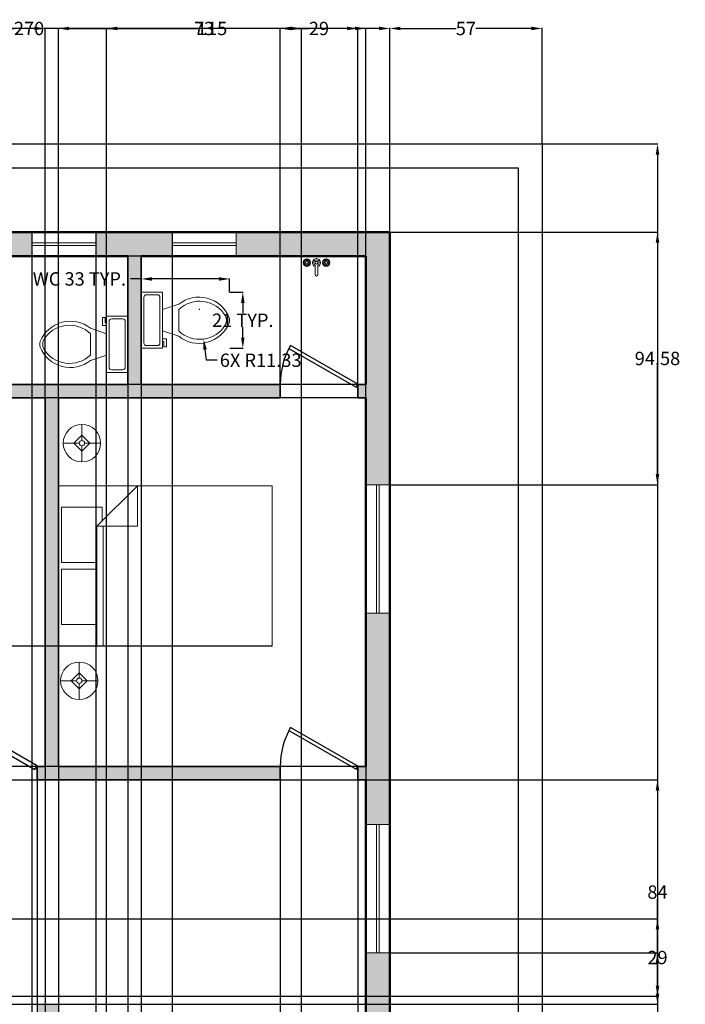
# Model space of a CAD drawing. Units: inches. Extents: x 882 to 1363, y 890 to 1847.
# Tile 9 of 9: x 1114 to 1363, y 1479 to 1847. Entities that reach past the tile are written whole.
import ezdxf

# ---------------------------------------------------------------- set-up
doc = ezdxf.new("R2010")
doc.units = ezdxf.units.IN
doc.header["$MEASUREMENT"] = 0
for name, color, linetype, lineweight in [('A-ANNO-DIMS', 2, 'Continuous', 18), ('C-PROP', 7, 'Continuous', 25), ('doors', 3, 'Continuous', 25), ('furniture', 10, 'Continuous', 18), ('inner wall', 50, 'Continuous', 35), ('outer wall', 40, 'Continuous', 50), ('sanitary', 231, 'Continuous', 18), ('ventilator', 130, 'Continuous', 18), ('windows', 226, 'Continuous', 18)]:
    doc.layers.add(name, color=color, linetype=linetype, lineweight=lineweight)
doc.layers.add('A-WALL-PATT', color=251, linetype='Continuous', lineweight=13, true_color=0x636466)
doc.styles.get("Standard").update_dxf_attribs({"font": 'arial.ttf'})
doc.dimstyles.get("Standard").update_dxf_attribs({"dimtxt": 5, "dimasz": 4, "dimexe": 0.18, "dimexo": 0.0625, "dimgap": 0.09, "dimtad": 0, "dimtih": 1, "dimtoh": 1, "dimdec": 1, "dimzin": 0, "dimdsep": 46, "dimlunit": 3, "dimtxsty": 'Standard', "dimcen": 0.09, "dimadec": 0, "dimazin": 0, "dimtfac": 1, "dimtdec": 1, "dimtofl": 0, "dimtmove": 0, "dimatfit": 3, "dimfxl": 1, "dimtolj": 1, "dimtzin": 0, "dimarcsym": 0})

# ---------------------------------------------------------------- blocks, each defined once
blk = doc.blocks.new('*U3')
for p, q in [((0, 0), (0, 6)), ((40, 0), (40, 6))]:
    blk.add_line(p, q)
blk.add_lwpolyline([(0, 0), (34.64, -20), (35.52, -18.48), (0.87, 1.52)], close=True)
blk.add_arc((0, 0), 40, 330, 0)
blk = doc.blocks.new('Toilet - top')
for p, q in [((9.5, -6), (9.5, -2)), ((-10, -8.5), (-8, -8.5)), ((-10, -9.5), (-10, -8.5)), ((-7, -9.5), (-10, -9.5)), ((-8, -8.5), (-8, -8)), ((-7, -8), (-7, -9.5)), ((-4, -8), (-6, -14)), ((4, -8), (6, -14)), ((4, -14), (-4, -14))]:
    blk.add_line(p, q)
blk.add_lwpolyline([(10.5, -8), (10.5, 0), (-10.5, 0), (-10.5, -8)], close=True)
for points in [[(-9.5, -2), (-9.5, -6)], [(8.5, -1), (-8.5, -1)], [(-8.5, -7), (8.5, -7)]]:
    blk.add_lwpolyline(points)
for centre, radius, start, end in [((-8.62, -1.88), 0.884, 81.8699, 188.1301), ((8.62, -1.88), 0.884, 351.8699, 98.1301), ((-8.62, -6.12), 0.884, 171.8699, 278.1301), ((8.62, -6.12), 0.884, 261.8699, 8.1301), ((3.52, -21.58), 12.17, 141.4691, 247.9714), ((4.2, -21.82), 11.33, 136.3677, 238.9468), ((-3.52, -21.58), 12.17, 292.0284, 38.5307), ((-4.2, -21.82), 11.33, 301.053, 43.6321), ((0, -27.88), 4, 245.7318, 294.2682), ((0, -29), 4, 254.8605, 285.1395)]:
    blk.add_arc(centre, radius, start, end)
blk = doc.blocks.new('Faucet - Bathroom top')
for p, q in [((-4.107, 0.125), (-4.375, 0.125)), ((-3.75, 0.4788), (-3.75, 0.75)), ((-3.5, 0.482), (-3.5, 0.75)), ((-3.1461, 0.125), (-2.875, 0.125)), ((3.143, 0.125), (2.875, 0.125)), ((3.5, 0.4788), (3.5, 0.75)), ((3.75, 0.482), (3.75, 0.75)), ((4.1039, 0.125), (4.375, 0.125)), ((-4.1039, -0.125), (-4.375, -0.125)), ((-3.75, -0.4821), (-3.75, -0.75)), ((-3.5, -0.4789), (-3.5, -0.75)), ((-3.143, -0.125), (-2.875, -0.125)), ((-0.5, -0.8639), (-0.5, -4.5)), ((0.5, -4.5), (0.5, -0.8631)), ((3.1461, -0.125), (2.875, -0.125)), ((3.5, -0.4821), (3.5, -0.75)), ((3.75, -0.4789), (3.75, -0.75)), ((4.107, -0.125), (4.375, -0.125))]:
    blk.add_line(p, q)
for centre, radius in [((-3.625, 0), 1.375), ((-4.625, 0), 0.2795), ((-3.625, 0), 0.5), ((-3.625, 1), 0.2795), ((-2.625, 0), 0.2795), ((0, 0), 0.5), ((3.625, 0), 1.375), ((2.625, 0), 0.2795), ((3.625, 0), 0.5), ((3.625, 1), 0.2795), ((4.625, 0), 0.2795), ((-3.625, -1), 0.2795), ((3.625, -1), 0.2795)]:
    blk.add_circle(centre, radius)
for centre, radius, start, end in [((-3.625, 0), 1, 105.2407, 164.2093), ((-3.625, 0), 1, 16.44125, 74.07887), ((0, 0), 1.5, 289.6514, 250.3603), ((0, 0), 1, 300.3431, 239.7554), ((3.625, 0), 1, 106.12, 164.0884), ((3.625, 0), 1, 16.23422, 73.90469), ((-3.625, 0), 1, 196.2342, 253.9047), ((-3.625, 0), 1, 286.12, 344.0884), ((3.625, 0), 1, 196.4413, 254.0789), ((3.625, 0), 1, 285.2407, 344.2093), ((0, -4.5), 0.5, 180, 0)]:
    blk.add_arc(centre, radius, start, end)
blk = doc.blocks.new('Bed - Queen')
for p, q in [((0, -80.00003), (0, 0)), ((0, 0), (59.99999, 0)), ((59.99999, 0), (59.99999, -80.00003)), ((7.99999, -1.2), (28.79998, -1.2)), ((7.99999, -14.4), (7.99999, -1.2)), ((28.79998, -1.2), (28.79998, -14.4)), ((31.19999, -1.2), (51.99999, -1.2)), ((31.19999, -14.4), (31.19999, -1.2)), ((51.99999, -1.2), (51.99999, -16.4)), ((0, -14.4), (44.8, -14.4)), ((59.99999, -29.6), (44.8, -14.4)), ((44.8, -14.4), (44.8, -29.6)), ((44.8, -16.8), (0, -16.8)), ((51.99999, -16.4), (46.79936, -16.4)), ((44.8, -29.6), (59.99999, -29.6)), ((59.99999, -80.00003), (0, -80.00003))]:
    blk.add_line(p, q)
blk = doc.blocks.new('Lamp - Table')
for p, q in [((0, 7), (0, 1)), ((-1, 0), (-7, 0)), ((0, 3), (-3, 0)), ((-3, 0), (0, -3)), ((3, 0), (0, 3)), ((0, -3), (3, 0)), ((1, 0), (7, 0)), ((0, -1), (0, -7))]:
    blk.add_line(p, q)
for radius in [7, 1]:
    blk.add_circle((0, 0), radius)
blk = doc.blocks.new('WIN-48IN-9IN')
for p, q in [((4, 0), (4, 48)), ((5, 0), (5, 48))]:
    blk.add_line(p, q)
blk.add_lwpolyline([(0, 48), (9, 48), (9, 0), (0, 0)], close=True)
blk = doc.blocks.new('VENT-24IN-9IN')
for p, q in [((24, 5), (0, 5)), ((24, 4), (0, 4))]:
    blk.add_line(p, q)
blk.add_lwpolyline([(0, 9), (24, 9), (24, 0), (0, 0)], close=True)
blk = doc.blocks.new('*D19')
at = {"layer": 'A-ANNO-DIMS', "color": 0, "lineweight": -2, "transparency": 16777216}
for p, q in [((1159.84, 1745.31), (1159.84, 1750.39)), ((1192.89, 1745.31), (1192.89, 1750.39)), ((1159.84, 1750.21), (1155.84, 1750.21)), ((1188.89, 1750.21), (1163.84, 1750.21))]:
    blk.add_line(p, q, dxfattribs=at)
at = {"layer": 'A-ANNO-DIMS', "color": 0, "transparency": 16777216}
for points in [[(1163.84, 1750.87), (1163.84, 1749.54), (1159.84, 1750.21)], [(1188.89, 1750.87), (1188.89, 1749.54), (1192.89, 1750.21)]]:
    blk.add_solid(points, dxfattribs=at)
at = {"layer": 'Defpoints', "color": 0, "transparency": 16777216}
for p in [(1159.84, 1750.21), (1159.84, 1745.25), (1192.89, 1745.25)]:
    blk.add_point(p, dxfattribs=at)
at = {"layer": 'A-ANNO-DIMS', "color": 0, "transparency": 16777216, "insert": (1136.69, 1750.21), "char_height": 5, "attachment_point": 5}
blk.add_mtext('\\A1;WC 33 TYP.', dxfattribs=at)
blk = doc.blocks.new('*D20')
at = {"layer": 'A-ANNO-DIMS', "color": 0, "lineweight": -2, "transparency": 16777216}
for p, q in [((1192.95, 1745.25), (1198.02, 1745.25)), ((1197.84, 1741.25), (1197.84, 1737.35)), ((1197.84, 1728.25), (1197.84, 1732.15)), ((1192.95, 1724.25), (1198.02, 1724.25))]:
    blk.add_line(p, q, dxfattribs=at)
at = {"layer": 'A-ANNO-DIMS', "color": 0, "transparency": 16777216}
for points in [[(1197.18, 1741.25), (1198.51, 1741.25), (1197.84, 1745.25)], [(1197.18, 1728.25), (1198.51, 1728.25), (1197.84, 1724.25)]]:
    blk.add_solid(points, dxfattribs=at)
at = {"layer": 'Defpoints', "color": 0, "transparency": 16777216}
for p in [(1192.89, 1745.25), (1197.84, 1745.25), (1192.89, 1724.25)]:
    blk.add_point(p, dxfattribs=at)
at = {"layer": 'A-ANNO-DIMS', "color": 0, "transparency": 16777216, "insert": (1197.84, 1734.75), "char_height": 5, "attachment_point": 5}
blk.add_mtext('\\A1;21 TYP.', dxfattribs=at)
blk = doc.blocks.new('*D34')
at = {"layer": 'A-ANNO-DIMS', "color": 0, "lineweight": -2, "transparency": 16777216}
for p, q in [((1309.9, 1800.75), (1353.22, 1800.75)), ((1353.04, 1796.75), (1353.04, 1371.39)), ((1353.04, 940.75), (1353.04, 1366.11)), ((1309.9, 936.75), (1353.22, 936.75))]:
    blk.add_line(p, q, dxfattribs=at)
at = {"layer": 'A-ANNO-DIMS', "color": 0, "transparency": 16777216}
for points in [[(1352.38, 1796.75), (1353.71, 1796.75), (1353.04, 1800.75)], [(1352.38, 940.75), (1353.71, 940.75), (1353.04, 936.75)]]:
    blk.add_solid(points, dxfattribs=at)
at = {"layer": 'Defpoints', "color": 0, "transparency": 16777216}
for p in [(1309.84, 1800.75), (1353.04, 1800.75), (1309.84, 936.75)]:
    blk.add_point(p, dxfattribs=at)
at = {"layer": 'A-ANNO-DIMS', "color": 0, "transparency": 16777216, "insert": (1353.04, 1368.75), "char_height": 5, "attachment_point": 5}
blk.add_mtext('\\A1;864', dxfattribs=at)
blk = doc.blocks.new('*D35')
at = {"layer": 'A-ANNO-DIMS', "color": 0, "lineweight": -2, "transparency": 16777216}
for p, q in [((1252.84, 1767.81), (1252.84, 1844.13)), ((1256.84, 1843.95), (1277.67, 1843.95)), ((1305.84, 1843.95), (1285.01, 1843.95)), ((1309.84, 1800.81), (1309.84, 1844.13))]:
    blk.add_line(p, q, dxfattribs=at)
at = {"layer": 'A-ANNO-DIMS', "color": 0, "transparency": 16777216}
for points in [[(1256.84, 1844.62), (1256.84, 1843.29), (1252.84, 1843.95)], [(1305.84, 1844.62), (1305.84, 1843.29), (1309.84, 1843.95)]]:
    blk.add_solid(points, dxfattribs=at)
at = {"layer": 'Defpoints', "color": 0, "transparency": 16777216}
for p in [(1252.84, 1843.95), (1309.84, 1800.75), (1252.84, 1767.75)]:
    blk.add_point(p, dxfattribs=at)
at = {"layer": 'A-ANNO-DIMS', "color": 0, "transparency": 16777216, "insert": (1281.34, 1843.95), "char_height": 5, "attachment_point": 5}
blk.add_mtext('\\A1;57', dxfattribs=at)
blk = doc.blocks.new('*D39')
at = {"layer": 'A-ANNO-DIMS', "color": 0, "lineweight": -2, "transparency": 16777216}
for p, q in [((982.84, 1767.81), (982.84, 1844.13)), ((986.84, 1843.95), (1112.19, 1843.95)), ((1248.84, 1843.95), (1123.49, 1843.95)), ((1252.84, 1767.81), (1252.84, 1844.13))]:
    blk.add_line(p, q, dxfattribs=at)
at = {"layer": 'A-ANNO-DIMS', "color": 0, "transparency": 16777216}
for points in [[(986.84, 1844.62), (986.84, 1843.29), (982.84, 1843.95)], [(1248.84, 1844.62), (1248.84, 1843.29), (1252.84, 1843.95)]]:
    blk.add_solid(points, dxfattribs=at)
at = {"layer": 'Defpoints', "color": 0, "transparency": 16777216}
for p in [(1252.84, 1843.95), (982.84, 1767.75), (1252.84, 1767.75)]:
    blk.add_point(p, dxfattribs=at)
at = {"layer": 'A-ANNO-DIMS', "color": 0, "transparency": 16777216, "insert": (1117.84, 1843.95), "char_height": 5, "attachment_point": 5}
blk.add_mtext('\\A1;270', dxfattribs=at)
blk = doc.blocks.new('*D41')
at = {"layer": 'A-ANNO-DIMS', "color": 0, "lineweight": -2, "transparency": 16777216}
for p, q in [((1069.84, 1758.69), (1069.84, 893.37)), ((1154.84, 1758.69), (1154.84, 893.37)), ((1073.84, 893.55), (1108.65, 893.55)), ((1150.84, 893.55), (1116.03, 893.55))]:
    blk.add_line(p, q, dxfattribs=at)
at = {"layer": 'A-ANNO-DIMS', "color": 0, "transparency": 16777216}
for points in [[(1073.84, 894.21), (1073.84, 892.88), (1069.84, 893.55)], [(1150.84, 894.21), (1150.84, 892.88), (1154.84, 893.55)]]:
    blk.add_solid(points, dxfattribs=at)
at = {"layer": 'Defpoints', "color": 0, "transparency": 16777216}
for p in [(1069.84, 1758.75), (1154.84, 1758.75), (1154.84, 893.55)]:
    blk.add_point(p, dxfattribs=at)
at = {"layer": 'A-ANNO-DIMS', "color": 0, "transparency": 16777216, "insert": (1112.34, 893.55), "char_height": 5, "attachment_point": 5}
blk.add_mtext('\\A1;85', dxfattribs=at)
blk = doc.blocks.new('*D42')
at = {"layer": 'A-ANNO-DIMS', "color": 0, "lineweight": -2, "transparency": 16777216}
for p, q in [((1159.84, 1710.69), (1159.84, 893.37)), ((1243.84, 1705.69), (1243.84, 893.37)), ((1163.84, 893.55), (1198.17, 893.55)), ((1239.84, 893.55), (1205.5, 893.55))]:
    blk.add_line(p, q, dxfattribs=at)
at = {"layer": 'A-ANNO-DIMS', "color": 0, "transparency": 16777216}
for points in [[(1163.84, 894.21), (1163.84, 892.88), (1159.84, 893.55)], [(1239.84, 894.21), (1239.84, 892.88), (1243.84, 893.55)]]:
    blk.add_solid(points, dxfattribs=at)
at = {"layer": 'Defpoints', "color": 0, "transparency": 16777216}
for p in [(1159.84, 1710.75), (1243.84, 1705.75), (1243.84, 893.55)]:
    blk.add_point(p, dxfattribs=at)
at = {"layer": 'A-ANNO-DIMS', "color": 0, "transparency": 16777216, "insert": (1201.84, 893.55), "char_height": 5, "attachment_point": 5}
blk.add_mtext('\\A1;84', dxfattribs=at)
blk = doc.blocks.new('*D43')
at = {"layer": 'A-ANNO-DIMS', "color": 0, "lineweight": -2, "transparency": 16777216}
for p, q in [((1243.78, 1758.75), (906.46, 1758.75)), ((906.64, 1754.75), (906.64, 1737.39)), ((906.64, 1714.75), (906.64, 1732.11)), ((1243.78, 1710.75), (906.46, 1710.75))]:
    blk.add_line(p, q, dxfattribs=at)
at = {"layer": 'A-ANNO-DIMS', "color": 0, "transparency": 16777216}
for points in [[(905.97, 1754.75), (907.3, 1754.75), (906.64, 1758.75)], [(905.97, 1714.75), (907.3, 1714.75), (906.64, 1710.75)]]:
    blk.add_solid(points, dxfattribs=at)
at = {"layer": 'Defpoints', "color": 0, "transparency": 16777216}
for p in [(1243.84, 1758.75), (906.64, 1710.75), (1243.84, 1710.75)]:
    blk.add_point(p, dxfattribs=at)
at = {"layer": 'A-ANNO-DIMS', "color": 0, "transparency": 16777216, "insert": (906.64, 1734.75), "char_height": 5, "attachment_point": 5}
blk.add_mtext('\\A1;48', dxfattribs=at)
blk = doc.blocks.new('*D44')
at = {"layer": 'A-ANNO-DIMS', "color": 0, "lineweight": -2, "transparency": 16777216}
for p, q in [((1243.78, 1705.75), (906.46, 1705.75)), ((906.64, 1701.75), (906.64, 1639.39)), ((906.64, 1571.75), (906.64, 1634.1)), ((1243.78, 1567.75), (906.46, 1567.75))]:
    blk.add_line(p, q, dxfattribs=at)
at = {"layer": 'A-ANNO-DIMS', "color": 0, "transparency": 16777216}
for points in [[(905.97, 1701.75), (907.3, 1701.75), (906.64, 1705.75)], [(905.97, 1571.75), (907.3, 1571.75), (906.64, 1567.75)]]:
    blk.add_solid(points, dxfattribs=at)
at = {"layer": 'Defpoints', "color": 0, "transparency": 16777216}
for p in [(1243.84, 1705.75), (906.64, 1567.75), (1243.84, 1567.75)]:
    blk.add_point(p, dxfattribs=at)
at = {"layer": 'A-ANNO-DIMS', "color": 0, "transparency": 16777216, "insert": (906.64, 1636.75), "char_height": 5, "attachment_point": 5}
blk.add_mtext('\\A1;138', dxfattribs=at)
blk = doc.blocks.new('*D45')
at = {"layer": 'A-ANNO-DIMS', "color": 0, "lineweight": -2, "transparency": 16777216}
for p, q in [((1128.84, 1567.81), (1128.84, 1844.13)), ((1132.84, 1843.95), (1180.94, 1843.95)), ((1239.84, 1843.95), (1191.74, 1843.95)), ((1243.84, 1567.81), (1243.84, 1844.13))]:
    blk.add_line(p, q, dxfattribs=at)
at = {"layer": 'A-ANNO-DIMS', "color": 0, "transparency": 16777216}
for points in [[(1132.84, 1844.62), (1132.84, 1843.29), (1128.84, 1843.95)], [(1239.84, 1844.62), (1239.84, 1843.29), (1243.84, 1843.95)]]:
    blk.add_solid(points, dxfattribs=at)
at = {"layer": 'Defpoints', "color": 0, "transparency": 16777216}
for p in [(1243.84, 1843.95), (1128.84, 1567.75), (1243.84, 1567.75)]:
    blk.add_point(p, dxfattribs=at)
at = {"layer": 'A-ANNO-DIMS', "color": 0, "transparency": 16777216, "insert": (1186.34, 1843.95), "char_height": 5, "attachment_point": 5}
blk.add_mtext('\\A1;115', dxfattribs=at)
blk = doc.blocks.new('*D46')
at = {"layer": 'A-ANNO-DIMS', "color": 0, "lineweight": -2, "transparency": 16777216}
for p, q in [((991.84, 1567.81), (991.84, 1844.13)), ((995.84, 1843.95), (1052.49, 1843.95)), ((1119.84, 1843.95), (1063.19, 1843.95)), ((1123.84, 1567.81), (1123.84, 1844.13))]:
    blk.add_line(p, q, dxfattribs=at)
at = {"layer": 'A-ANNO-DIMS', "color": 0, "transparency": 16777216}
for points in [[(995.84, 1844.62), (995.84, 1843.29), (991.84, 1843.95)], [(1119.84, 1844.62), (1119.84, 1843.29), (1123.84, 1843.95)]]:
    blk.add_solid(points, dxfattribs=at)
at = {"layer": 'Defpoints', "color": 0, "transparency": 16777216}
for p in [(1123.84, 1843.95), (991.84, 1567.75), (1123.84, 1567.75)]:
    blk.add_point(p, dxfattribs=at)
at = {"layer": 'A-ANNO-DIMS', "color": 0, "transparency": 16777216, "insert": (1057.84, 1843.95), "char_height": 5, "attachment_point": 5}
blk.add_mtext('\\A1;132', dxfattribs=at)
blk = doc.blocks.new('*D47')
at = {"layer": 'A-ANNO-DIMS', "color": 0, "lineweight": -2, "transparency": 16777216}
for p, q in [((1123.84, 1567.69), (1123.84, 893.37)), ((1128.84, 1567.69), (1128.84, 893.37)), ((1119.84, 893.55), (1115.84, 893.55)), ((1132.84, 893.55), (1136.84, 893.55))]:
    blk.add_line(p, q, dxfattribs=at)
at = {"layer": 'A-ANNO-DIMS', "color": 0, "transparency": 16777216}
for points in [[(1119.84, 894.21), (1119.84, 892.88), (1123.84, 893.55)], [(1132.84, 894.21), (1132.84, 892.88), (1128.84, 893.55)]]:
    blk.add_solid(points, dxfattribs=at)
at = {"layer": 'Defpoints', "color": 0, "transparency": 16777216}
for p in [(1123.84, 1567.75), (1128.84, 1567.75), (1128.84, 893.55)]:
    blk.add_point(p, dxfattribs=at)
at = {"layer": 'A-ANNO-DIMS', "color": 0, "transparency": 16777216, "insert": (1126.34, 893.55), "char_height": 5, "attachment_point": 5}
blk.add_mtext('\\A1;5', dxfattribs=at)
blk = doc.blocks.new('*D48')
at = {"layer": 'A-ANNO-DIMS', "color": 0, "lineweight": -2, "transparency": 16777216}
for p, q in [((1084.84, 1562.69), (1084.84, 893.37)), ((1120.84, 1562.69), (1120.84, 893.37)), ((1088.84, 893.55), (1099.17, 893.55)), ((1116.84, 893.55), (1106.51, 893.55))]:
    blk.add_line(p, q, dxfattribs=at)
at = {"layer": 'A-ANNO-DIMS', "color": 0, "transparency": 16777216}
for points in [[(1088.84, 894.21), (1088.84, 892.88), (1084.84, 893.55)], [(1116.84, 894.21), (1116.84, 892.88), (1120.84, 893.55)]]:
    blk.add_solid(points, dxfattribs=at)
at = {"layer": 'Defpoints', "color": 0, "transparency": 16777216}
for p in [(1084.84, 1562.75), (1120.84, 1562.75), (1120.84, 893.55)]:
    blk.add_point(p, dxfattribs=at)
at = {"layer": 'A-ANNO-DIMS', "color": 0, "transparency": 16777216, "insert": (1102.84, 893.55), "char_height": 5, "attachment_point": 5}
blk.add_mtext('\\A1;36', dxfattribs=at)
blk = doc.blocks.new('*D49')
at = {"layer": 'A-ANNO-DIMS', "color": 0, "lineweight": -2, "transparency": 16777216}
for p, q in [((1211.84, 1562.69), (1211.84, 893.37)), ((1240.84, 1562.69), (1240.84, 893.37)), ((1215.84, 893.55), (1222.62, 893.55)), ((1236.84, 893.55), (1230.06, 893.55))]:
    blk.add_line(p, q, dxfattribs=at)
at = {"layer": 'A-ANNO-DIMS', "color": 0, "transparency": 16777216}
for points in [[(1215.84, 894.21), (1215.84, 892.88), (1211.84, 893.55)], [(1236.84, 894.21), (1236.84, 892.88), (1240.84, 893.55)]]:
    blk.add_solid(points, dxfattribs=at)
at = {"layer": 'Defpoints', "color": 0, "transparency": 16777216}
for p in [(1211.84, 1562.75), (1240.84, 1562.75), (1240.84, 893.55)]:
    blk.add_point(p, dxfattribs=at)
at = {"layer": 'A-ANNO-DIMS', "color": 0, "transparency": 16777216, "insert": (1226.34, 893.55), "char_height": 5, "attachment_point": 5}
blk.add_mtext('\\A1;29', dxfattribs=at)
blk = doc.blocks.new('*D50')
at = {"layer": 'A-ANNO-DIMS', "color": 0, "lineweight": -2, "transparency": 16777216}
for p, q in [((1252.9, 1767.75), (1353.22, 1767.75)), ((1353.04, 1763.75), (1353.04, 1723.1)), ((1353.04, 1677.17), (1353.04, 1717.82)), ((1252.9, 1673.17), (1353.22, 1673.17))]:
    blk.add_line(p, q, dxfattribs=at)
at = {"layer": 'A-ANNO-DIMS', "color": 0, "transparency": 16777216}
for points in [[(1352.38, 1763.75), (1353.71, 1763.75), (1353.04, 1767.75)], [(1352.38, 1677.17), (1353.71, 1677.17), (1353.04, 1673.17)]]:
    blk.add_solid(points, dxfattribs=at)
at = {"layer": 'Defpoints', "color": 0, "transparency": 16777216}
for p in [(1252.84, 1767.75), (1252.84, 1673.17), (1353.04, 1673.17)]:
    blk.add_point(p, dxfattribs=at)
at = {"layer": 'A-ANNO-DIMS', "color": 0, "transparency": 16777216, "insert": (1353.04, 1720.46), "char_height": 5, "attachment_point": 5}
blk.add_mtext('\\A1;94.58', dxfattribs=at)
blk = doc.blocks.new('*D52')
at = {"layer": 'A-ANNO-DIMS', "color": 0, "lineweight": -2, "transparency": 16777216}
for p, q in [((1048.84, 1767.69), (1048.84, 893.37)), ((1118.86, 1767.69), (1118.86, 893.37)), ((1052.84, 893.55), (1075.83, 893.55)), ((1114.86, 893.55), (1091.87, 893.55))]:
    blk.add_line(p, q, dxfattribs=at)
at = {"layer": 'A-ANNO-DIMS', "color": 0, "transparency": 16777216}
for points in [[(1052.84, 894.21), (1052.84, 892.88), (1048.84, 893.55)], [(1114.86, 894.21), (1114.86, 892.88), (1118.86, 893.55)]]:
    blk.add_solid(points, dxfattribs=at)
at = {"layer": 'Defpoints', "color": 0, "transparency": 16777216}
for p in [(1048.84, 1767.75), (1118.86, 1767.75), (1118.86, 893.55)]:
    blk.add_point(p, dxfattribs=at)
at = {"layer": 'A-ANNO-DIMS', "color": 0, "transparency": 16777216, "insert": (1083.85, 893.55), "char_height": 5, "attachment_point": 5}
blk.add_mtext('\\A1;70.01', dxfattribs=at)
blk = doc.blocks.new('*D53')
at = {"layer": 'A-ANNO-DIMS', "color": 0, "lineweight": -2, "transparency": 16777216}
for p, q in [((1142.86, 1767.69), (1142.86, 893.37)), ((1171.41, 1767.69), (1171.41, 893.37)), ((1138.86, 893.55), (1134.86, 893.55)), ((1175.41, 893.55), (1179.41, 893.55))]:
    blk.add_line(p, q, dxfattribs=at)
at = {"layer": 'A-ANNO-DIMS', "color": 0, "transparency": 16777216}
for points in [[(1138.86, 894.21), (1138.86, 892.88), (1142.86, 893.55)], [(1175.41, 894.21), (1175.41, 892.88), (1171.41, 893.55)]]:
    blk.add_solid(points, dxfattribs=at)
at = {"layer": 'Defpoints', "color": 0, "transparency": 16777216}
for p in [(1142.86, 1767.75), (1171.41, 1767.75), (1171.41, 893.55)]:
    blk.add_point(p, dxfattribs=at)
at = {"layer": 'A-ANNO-DIMS', "color": 0, "transparency": 16777216, "insert": (1157.14, 893.55), "char_height": 5, "attachment_point": 5}
blk.add_mtext('\\A1;28.554', dxfattribs=at)
blk = doc.blocks.new('*D56')
at = {"layer": 'A-ANNO-DIMS', "color": 0, "lineweight": -2, "transparency": 16777216}
for p, q in [((991.9, 1562.75), (1353.22, 1562.75)), ((1353.04, 1558.75), (1353.04, 1523.39)), ((1353.04, 1482.75), (1353.04, 1518.11)), ((991.9, 1478.75), (1353.22, 1478.75))]:
    blk.add_line(p, q, dxfattribs=at)
at = {"layer": 'A-ANNO-DIMS', "color": 0, "transparency": 16777216}
for points in [[(1352.38, 1558.75), (1353.71, 1558.75), (1353.04, 1562.75)], [(1352.38, 1482.75), (1353.71, 1482.75), (1353.04, 1478.75)]]:
    blk.add_solid(points, dxfattribs=at)
at = {"layer": 'Defpoints', "color": 0, "transparency": 16777216}
for p in [(991.84, 1562.75), (991.84, 1478.75), (1353.04, 1478.75)]:
    blk.add_point(p, dxfattribs=at)
at = {"layer": 'A-ANNO-DIMS', "color": 0, "transparency": 16777216, "insert": (1353.04, 1520.75), "char_height": 5, "attachment_point": 5}
blk.add_mtext('\\A1;84', dxfattribs=at)
blk = doc.blocks.new('*D60')
at = {"layer": 'A-ANNO-DIMS', "color": 0, "lineweight": -2, "transparency": 16777216}
for p, q in [((1050.9, 1510.75), (1353.22, 1510.75)), ((1353.04, 1506.75), (1353.04, 1498.89)), ((1353.04, 1485.75), (1353.04, 1493.61)), ((1050.9, 1481.75), (1353.22, 1481.75))]:
    blk.add_line(p, q, dxfattribs=at)
at = {"layer": 'A-ANNO-DIMS', "color": 0, "transparency": 16777216}
for points in [[(1352.38, 1506.75), (1353.71, 1506.75), (1353.04, 1510.75)], [(1352.38, 1485.75), (1353.71, 1485.75), (1353.04, 1481.75)]]:
    blk.add_solid(points, dxfattribs=at)
at = {"layer": 'Defpoints', "color": 0, "transparency": 16777216}
for p in [(1050.84, 1510.75), (1050.84, 1481.75), (1353.04, 1481.75)]:
    blk.add_point(p, dxfattribs=at)
at = {"layer": 'A-ANNO-DIMS', "color": 0, "transparency": 16777216, "insert": (1353.04, 1496.25), "char_height": 5, "attachment_point": 5}
blk.add_mtext('\\A1;29', dxfattribs=at)
blk = doc.blocks.new('*D78')
at = {"layer": 'A-ANNO-DIMS', "color": 0, "lineweight": -2, "transparency": 16777216}
for p, q in [((1146.84, 1274.81), (1146.84, 1844.13)), ((1150.84, 1843.95), (1179.69, 1843.95)), ((1215.84, 1843.95), (1186.99, 1843.95)), ((1219.84, 1274.81), (1219.84, 1844.13))]:
    blk.add_line(p, q, dxfattribs=at)
at = {"layer": 'A-ANNO-DIMS', "color": 0, "transparency": 16777216}
for points in [[(1150.84, 1844.62), (1150.84, 1843.29), (1146.84, 1843.95)], [(1215.84, 1844.62), (1215.84, 1843.29), (1219.84, 1843.95)]]:
    blk.add_solid(points, dxfattribs=at)
at = {"layer": 'Defpoints', "color": 0, "transparency": 16777216}
for p in [(1219.84, 1843.95), (1146.84, 1274.75), (1219.84, 1274.75)]:
    blk.add_point(p, dxfattribs=at)
at = {"layer": 'A-ANNO-DIMS', "color": 0, "transparency": 16777216, "insert": (1183.34, 1843.95), "char_height": 5, "attachment_point": 5}
blk.add_mtext('\\A1;73', dxfattribs=at)
blk = doc.blocks.new('*D80')
at = {"layer": 'A-ANNO-DIMS', "color": 0, "lineweight": -2, "transparency": 16777216}
for p, q in [((1252.9, 1498.03), (1353.22, 1498.03)), ((1353.04, 1494.03), (1353.04, 1447.23)), ((1353.04, 1395.14), (1353.04, 1441.94)), ((1252.9, 1391.14), (1353.22, 1391.14))]:
    blk.add_line(p, q, dxfattribs=at)
at = {"layer": 'A-ANNO-DIMS', "color": 0, "transparency": 16777216}
for points in [[(1352.38, 1494.03), (1353.71, 1494.03), (1353.04, 1498.03)], [(1352.38, 1395.14), (1353.71, 1395.14), (1353.04, 1391.14)]]:
    blk.add_solid(points, dxfattribs=at)
at = {"layer": 'Defpoints', "color": 0, "transparency": 16777216}
for p in [(1252.84, 1498.03), (1353.04, 1498.03), (1252.84, 1391.14)]:
    blk.add_point(p, dxfattribs=at)
at = {"layer": 'A-ANNO-DIMS', "color": 0, "transparency": 16777216, "insert": (1353.04, 1444.58), "char_height": 5, "attachment_point": 5}
blk.add_mtext('\\A1;106.89', dxfattribs=at)
blk = doc.blocks.new('*D86')
at = {"layer": 'A-ANNO-DIMS', "color": 0, "lineweight": -2, "transparency": 16777216}
for p, q in [((1211.84, 1710.81), (1211.84, 1844.13)), ((1215.84, 1843.95), (1222.62, 1843.95)), ((1236.84, 1843.95), (1230.06, 1843.95)), ((1240.84, 1710.81), (1240.84, 1844.13))]:
    blk.add_line(p, q, dxfattribs=at)
at = {"layer": 'A-ANNO-DIMS', "color": 0, "transparency": 16777216}
for points in [[(1215.84, 1844.62), (1215.84, 1843.29), (1211.84, 1843.95)], [(1236.84, 1844.62), (1236.84, 1843.29), (1240.84, 1843.95)]]:
    blk.add_solid(points, dxfattribs=at)
at = {"layer": 'Defpoints', "color": 0, "transparency": 16777216}
for p in [(1240.84, 1843.95), (1211.84, 1710.75), (1240.84, 1710.75)]:
    blk.add_point(p, dxfattribs=at)
at = {"layer": 'A-ANNO-DIMS', "color": 0, "transparency": 16777216, "insert": (1226.34, 1843.95), "char_height": 5, "attachment_point": 5}
blk.add_mtext('\\A1;29', dxfattribs=at)
blk = doc.blocks.new('*D88')
at = {"layer": 'A-ANNO-DIMS', "color": 0, "lineweight": -2, "transparency": 16777216}
for p, q in [((1128.84, 1567.69), (1128.84, 893.37)), ((1211.84, 1562.69), (1211.84, 893.37)), ((1132.84, 893.55), (1166.66, 893.55)), ((1207.84, 893.55), (1174.01, 893.55))]:
    blk.add_line(p, q, dxfattribs=at)
at = {"layer": 'A-ANNO-DIMS', "color": 0, "transparency": 16777216}
for points in [[(1132.84, 894.21), (1132.84, 892.88), (1128.84, 893.55)], [(1207.84, 894.21), (1207.84, 892.88), (1211.84, 893.55)]]:
    blk.add_solid(points, dxfattribs=at)
at = {"layer": 'Defpoints', "color": 0, "transparency": 16777216}
for p in [(1128.84, 1567.75), (1211.84, 1562.75), (1211.84, 893.55)]:
    blk.add_point(p, dxfattribs=at)
at = {"layer": 'A-ANNO-DIMS', "color": 0, "transparency": 16777216, "insert": (1170.34, 893.55), "char_height": 5, "attachment_point": 5}
blk.add_mtext('\\A1;83', dxfattribs=at)
blk = doc.blocks.new('*D91')
at = {"layer": 'A-ANNO-DIMS', "color": 0, "lineweight": -2, "transparency": 16777216}
for p, q in [((1208.78, 1612.84), (906.46, 1612.84)), ((906.64, 1608.84), (906.64, 1592.94)), ((906.64, 1571.75), (906.64, 1587.65)), ((1211.78, 1567.75), (906.46, 1567.75))]:
    blk.add_line(p, q, dxfattribs=at)
at = {"layer": 'A-ANNO-DIMS', "color": 0, "transparency": 16777216}
for points in [[(905.97, 1608.84), (907.3, 1608.84), (906.64, 1612.84)], [(905.97, 1571.75), (907.3, 1571.75), (906.64, 1567.75)]]:
    blk.add_solid(points, dxfattribs=at)
at = {"layer": 'Defpoints', "color": 0, "transparency": 16777216}
for p in [(1208.84, 1612.84), (906.64, 1567.75), (1211.84, 1567.75)]:
    blk.add_point(p, dxfattribs=at)
at = {"layer": 'A-ANNO-DIMS', "color": 0, "transparency": 16777216, "insert": (906.64, 1590.29), "char_height": 5, "attachment_point": 5}
blk.add_mtext('\\A1;45.09', dxfattribs=at)
blk = doc.blocks.new('*D96')
at = {"layer": 'A-ANNO-DIMS', "color": 0, "lineweight": -2, "transparency": 16777216}
for p, q in [((1181.57, 1738.95), (1181.75, 1738.95)), ((1181.66, 1738.86), (1181.66, 1739.04)), ((1184.23, 1719.79), (1183.7, 1723.76)), ((1188.23, 1719.79), (1184.23, 1719.79))]:
    blk.add_line(p, q, dxfattribs=at)
at = {"layer": 'A-ANNO-DIMS', "color": 0, "transparency": 16777216}
blk.add_solid([(1184.36, 1723.85), (1183.04, 1723.67), (1183.17, 1727.72)], dxfattribs=at)
at = {"layer": 'Defpoints', "color": 0, "transparency": 16777216}
for p in [(1181.66, 1738.95), (1183.17, 1727.72)]:
    blk.add_point(p, dxfattribs=at)
at = {"layer": 'A-ANNO-DIMS', "color": 0, "transparency": 16777216, "insert": (1204.54, 1719.79), "char_height": 5, "attachment_point": 5}
blk.add_mtext('\\A1;6X R11.33', dxfattribs=at)

msp = doc.modelspace()

# ---------------------------------------------------------------- hatches: boundary and pattern name
at = {"layer": 'A-WALL-PATT'}
h = msp.add_hatch(color=256, dxfattribs=at)
h.dxf.hatch_style = 1
h.paths.add_polyline_path([(1050.8388, 1481.7495), (1050.8388, 1478.7495), (1084.8388, 1478.7495), (1084.8388, 1473.7495), (991.8388, 1473.7495), (991.8388, 1361.0778), (982.8388, 1361.0778), (982.8388, 1556.1531), (991.8388, 1556.1531), (991.8388, 1478.7495), (1045.8388, 1478.7495), (1045.8388, 1481.7479), (1045.4161, 1481.7477), (1030.9055, 1506.8563), (1032.004, 1507.4911), (1046.5146, 1482.3825), (1045.4161, 1481.7477), (1045.8388, 1481.7479), (1045.8388, 1481.7495)])
h.paths.add_polyline_path([(1128.8388, 1478.7495), (1120.8388, 1478.7495), (1120.8388, 1473.7495), (1123.8388, 1473.7495), (1123.8388, 1353.7495), (991.8388, 1353.7495), (991.8388, 1361.0778), (982.8388, 1361.0778), (982.8388, 1337.3333), (991.8388, 1337.3333), (991.8388, 1348.7495), (1128.8388, 1348.7495)])
h.paths.add_polyline_path([(1118.8585, 1767.7495), (1048.8447, 1767.7495), (1048.8447, 1758.7495), (1064.8388, 1758.7495), (1069.8388, 1758.7495), (1118.8585, 1758.7495)])
h.paths.add_polyline_path([(1171.4129, 1767.7495), (1142.8585, 1767.7495), (1142.8585, 1758.7495), (1154.8388, 1758.7495), (1154.8388, 1710.7495), (1069.8388, 1710.7495), (1069.8388, 1713.7495), (1064.8388, 1713.7495), (1064.8388, 1705.7495), (1123.8388, 1705.7495), (1123.8388, 1567.7495), (1120.8388, 1567.7495), (1120.8388, 1562.7495), (1123.8388, 1562.7495), (1211.8388, 1562.7495), (1211.8388, 1567.7495), (1128.8388, 1567.7495), (1128.8388, 1705.7495), (1211.8388, 1705.7495), (1211.8388, 1710.7495), (1159.8388, 1710.7495), (1159.8388, 1758.7495), (1171.4129, 1758.7495)])
h.paths.add_polyline_path([(1252.8388, 1767.7495), (1195.4129, 1767.7495), (1195.4129, 1758.7495), (1243.8388, 1758.7495), (1243.8388, 1710.7495), (1240.8388, 1710.7495), (1240.8388, 1706.4648), (1240.8388, 1705.7495), (1243.8388, 1705.7495), (1243.8388, 1673.1735), (1252.8388, 1673.1735)])
h.paths.add_polyline_path([(1252.8388, 1625.1735), (1243.8388, 1625.1735), (1243.8388, 1567.7495), (1240.8388, 1567.7495), (1240.8388, 1562.7495), (1243.8388, 1562.7495), (1243.8388, 1546.029), (1252.8388, 1546.029)])
h.paths.add_polyline_path([(1252.8388, 1498.029), (1243.8388, 1498.029), (1243.8388, 1391.1399), (1252.8388, 1391.1399)])
h.paths.add_polyline_path([(1252.8388, 1179.8561), (1243.8388, 1179.8561), (1243.8388, 1149.7495), (1219.8388, 1149.7495), (1219.8388, 1145.3111), (1219.8388, 1144.7495), (1252.8388, 1144.7495)])
h.paths.add_polyline_path([(1252.8388, 1277.7495), (1243.8388, 1277.7495), (1243.8388, 1274.7495), (1219.8388, 1274.7495), (1219.8388, 1269.7495), (1243.8388, 1269.7495), (1243.8388, 1227.8561), (1252.8388, 1227.8561)])
h.paths.add_polyline_path([(1252.8388, 1343.1399), (1243.8388, 1343.1399), (1243.8388, 1313.7495), (1248.3388, 1313.7495), (1252.8388, 1313.7495)])
h.paths.add_polyline_path([(1146.8388, 1274.7495), (1112.8388, 1274.7495), (1112.8388, 1106.7495), (1106.7761, 1106.7495), (1106.7761, 1101.7495), (1117.8388, 1101.7495), (1117.8388, 1144.7495), (1159.8388, 1144.7495), (1159.8388, 1149.7495), (1117.8388, 1149.7495), (1117.8388, 1269.7495), (1146.8388, 1269.7495)])
h = msp.add_hatch(color=256, dxfattribs=at)
h.dxf.hatch_style = 1
h.paths.add_polyline_path([(1069.8388, 1758.7495), (1118.8585, 1758.7495), (1118.8585, 1767.7495), (1048.8447, 1767.7495), (1048.8447, 1758.7495), (1064.8388, 1758.7495), (1064.8388, 1742.7495), (1069.8388, 1742.7495)])

# ---------------------------------------------------------------- linework, layer by layer
at = {"layer": 'C-PROP'}
for points in [[(949.8388, 1800.7495), (1309.8388, 1800.7495), (1309.8388, 936.7495), (949.8388, 936.7495)], [(958.8388, 1791.7495), (1300.8388, 1791.7495), (1300.8388, 945.7495), (958.8388, 945.7495)]]:
    msp.add_lwpolyline(points, close=True, dxfattribs=at)
at = {"layer": 'inner wall'}
for p, q in [((1154.8388, 1758.7495), (1154.8388, 1710.7495)), ((1159.8388, 1758.7495), (1159.8388, 1710.7495)), ((1069.8388, 1710.7495), (1154.8388, 1710.7495)), ((1159.8388, 1710.7495), (1211.8388, 1710.7495)), ((1211.8388, 1710.7495), (1211.8388, 1705.7495)), ((1240.8388, 1710.7495), (1240.8388, 1705.7495)), ((1240.8388, 1710.7495), (1243.8388, 1710.7495)), ((1064.8388, 1705.7495), (1123.8388, 1705.7495)), ((1123.8388, 1567.7495), (1123.8388, 1705.7495)), ((1128.8388, 1705.7495), (1211.8388, 1705.7495)), ((1128.8388, 1567.7495), (1128.8388, 1705.7495)), ((1240.8388, 1705.7495), (1243.8388, 1705.7495)), ((1120.8388, 1562.7495), (1120.8388, 1567.7495)), ((1120.8388, 1567.7495), (1123.8388, 1567.7495)), ((1128.8388, 1567.7495), (1211.8388, 1567.7495)), ((1211.8388, 1567.7495), (1211.8388, 1562.7495)), ((1240.8388, 1567.7495), (1240.8388, 1562.7495)), ((1240.8388, 1567.7495), (1243.8388, 1567.7495)), ((1120.8388, 1562.7495), (1123.8388, 1562.7495)), ((1123.8388, 1562.7495), (1211.8388, 1562.7495)), ((1240.8388, 1562.7495), (1243.8388, 1562.7495))]:
    msp.add_line(p, q, dxfattribs=at)
at = {"layer": 'outer wall'}
for p, q in [((982.8388, 1767.7495), (1252.8388, 1767.7495)), ((1252.8388, 1767.7495), (1252.8388, 1313.7495)), ((1069.8388, 1758.7495), (1154.8388, 1758.7495)), ((1159.8388, 1758.7495), (1243.8388, 1758.7495)), ((1243.8388, 1758.7495), (1243.8388, 1710.7495)), ((1243.8388, 1705.7495), (1243.8388, 1567.7495)), ((1243.8388, 1562.7495), (1243.8388, 1313.7495))]:
    msp.add_line(p, q, dxfattribs=at)
at = {"layer": 'ventilator'}
for p, q in [((1142.8585, 1763.7495), (1118.8585, 1763.7495)), ((1142.8585, 1762.7495), (1118.8585, 1762.7495))]:
    msp.add_line(p, q, dxfattribs=at)
msp.add_lwpolyline([(1118.8585, 1767.7495), (1142.8585, 1767.7495), (1142.8585, 1758.7495), (1118.8585, 1758.7495)], close=True, dxfattribs=at)

# ---------------------------------------------------------------- block references
at = {"layer": 'doors', "rotation": 180}
for p, xscale, yscale, zscale in [((1240.8388, 1710.8148), 0.725, 0.725, 0.725), ((1120.8388, 1567.9495), 0.9, 0.9, 0.9), ((1240.8388, 1567.8122), 0.725, 0.725, 0.725)]:
    msp.add_blockref('*U3', p, dxfattribs=dict(at, xscale=xscale, yscale=yscale, zscale=zscale))
at = {"layer": 'furniture'}
for p in [(1137.6388, 1688.7495), (1136.6388, 1599.8306)]:
    msp.add_blockref('Lamp - Table', p, dxfattribs=at)
at = {"layer": 'furniture', "rotation": 90}
msp.add_blockref('Bed - Queen', (1128.8388, 1612.8355), dxfattribs=at)
at = {"layer": 'sanitary'}
msp.add_blockref('Faucet - Bathroom top', (1225.4236, 1756.3037), dxfattribs=at)
for p, rotation in [((1159.8388, 1734.7495), 90), ((1154.8388, 1725.7299), 270)]:
    msp.add_blockref('Toilet - top', p, dxfattribs=dict(at, rotation=rotation))
at = {"layer": 'ventilator'}
msp.add_blockref('VENT-24IN-9IN', (1171.413, 1758.75), dxfattribs=at)
at = {"layer": 'windows'}
for p in [(1243.839, 1625.1738), (1243.839, 1498.0292)]:
    msp.add_blockref('WIN-48IN-9IN', p, dxfattribs=at)

# ---------------------------------------------------------------- dimensions: what is measured, and where the dimension line sits
at = {"layer": 'A-ANNO-DIMS'}
for base, p1, p2, override, picture, middle in [((1252.8388, 1843.953), (982.8388, 1767.7495), (1252.8388, 1767.7495), {"dimdec": 0, "dimlfac": 1, "dimrnd": 0, "dimzin": 0, "dimdsep": 46, "dimlunit": 2}, '*D39', (1117.8388, 1843.953)), ((1123.8388, 1843.953), (991.8388, 1567.7495), (1123.8388, 1567.7495), {"dimdec": 0, "dimlfac": 1, "dimrnd": 0, "dimzin": 0, "dimdsep": 46, "dimlunit": 2}, '*D46', (1057.8388, 1843.953)), ((1243.8388, 1843.953), (1128.8388, 1567.7495), (1243.8388, 1567.7495), {"dimdec": 0, "dimlfac": 1, "dimrnd": 0, "dimzin": 0, "dimdsep": 46, "dimlunit": 2}, '*D45', (1186.3388, 1843.953)), ((1219.8388, 1843.953), (1146.8388, 1274.7495), (1219.8388, 1274.7495), {"dimdec": 0, "dimlfac": 1, "dimrnd": 0, "dimzin": 0, "dimdsep": 46, "dimlunit": 2}, '*D78', (1183.3388, 1843.953)), ((1240.8388, 1843.953), (1211.8388, 1710.7495), (1240.8388, 1710.7495), {"dimdec": 0, "dimlfac": 1, "dimrnd": 0, "dimzin": 0, "dimdsep": 46, "dimlunit": 2}, '*D86', (1226.3388, 1843.953)), ((1252.8388, 1843.953), (1309.8388, 1800.7495), (1252.8388, 1767.7495), {"dimdec": 0, "dimlfac": 1, "dimrnd": 0, "dimzin": 0, "dimdsep": 46, "dimlunit": 2}, '*D35', (1281.3388, 1843.953)), ((1118.8585, 893.546), (1048.8447, 1767.7495), (1118.8585, 1767.7495), {"dimdec": 2, "dimlfac": 1, "dimrnd": 0, "dimzin": 0, "dimdsep": 46, "dimlunit": 2}, '*D52', (1083.8516, 893.546)), ((1171.4129, 893.546), (1142.8585, 1767.7495), (1171.4129, 1767.7495), {"dimdec": 3, "dimlfac": 1, "dimrnd": 0, "dimzin": 0, "dimdsep": 46, "dimlunit": 2}, '*D53', (1157.1357, 893.546)), ((1154.8388, 893.546), (1069.8388, 1758.7495), (1154.8388, 1758.7495), {"dimdec": 0, "dimlfac": 1, "dimrnd": 0, "dimzin": 0, "dimdsep": 46, "dimlunit": 2}, '*D41', (1112.3388, 893.546)), ((1243.8388, 893.546), (1159.8388, 1710.7495), (1243.8388, 1705.7495), {"dimdec": 0, "dimlfac": 1, "dimrnd": 0, "dimzin": 0, "dimdsep": 46, "dimlunit": 2}, '*D42', (1201.8388, 893.546)), ((1128.8388, 893.546), (1123.8388, 1567.7495), (1128.8388, 1567.7495), {"dimdec": 0, "dimlfac": 1, "dimrnd": 0, "dimzin": 0, "dimdsep": 46, "dimlunit": 2}, '*D47', (1126.3388, 893.546)), ((1211.8388, 893.546), (1128.8388, 1567.7495), (1211.8388, 1562.7495), {"dimdec": 0, "dimlfac": 1, "dimrnd": 0, "dimzin": 0, "dimdsep": 46, "dimlunit": 2}, '*D88', (1170.3388, 893.546)), ((1120.8388, 893.546), (1084.8388, 1562.7495), (1120.8388, 1562.7495), {"dimdec": 0, "dimlfac": 1, "dimrnd": 0, "dimzin": 0, "dimdsep": 46, "dimlunit": 2}, '*D48', (1102.8388, 893.546)), ((1240.8388, 893.546), (1211.8388, 1562.7495), (1240.8388, 1562.7495), {"dimdec": 0, "dimlfac": 1, "dimrnd": 0, "dimzin": 0, "dimdsep": 46, "dimlunit": 2}, '*D49', (1226.3388, 893.546))]:
    dim = msp.add_linear_dim(base=base, p1=p1, p2=p2, dimstyle='Standard', override=override, dxfattribs=at)
    dim.commit()
    dim.dimension.update_dxf_attribs({"geometry": picture, "text_midpoint": middle})
for base, p1, p2, override, picture, middle in [((1353.0423, 1800.7495), (1309.8388, 936.7495), (1309.8388, 1800.7495), {"dimdec": 0, "dimlfac": 1, "dimrnd": 0, "dimzin": 0, "dimdsep": 46, "dimlunit": 2}, '*D34', (1353.0423, 1368.7495)), ((1353.0423, 1673.1735), (1252.8388, 1767.7495), (1252.8388, 1673.1735), {"dimdec": 2, "dimlfac": 1, "dimrnd": 0, "dimzin": 0, "dimdsep": 46, "dimlunit": 2}, '*D50', (1353.0423, 1720.4615)), ((906.6353, 1710.7495), (1243.8388, 1758.7495), (1243.8388, 1710.7495), {"dimdec": 0, "dimlfac": 1, "dimrnd": 0, "dimzin": 0, "dimdsep": 46, "dimlunit": 2}, '*D43', (906.6353, 1734.7495)), ((906.6353, 1567.7495), (1243.8388, 1705.7495), (1243.8388, 1567.7495), {"dimdec": 0, "dimlfac": 1, "dimrnd": 0, "dimzin": 0, "dimdsep": 46, "dimlunit": 2}, '*D44', (906.6353, 1636.7495)), ((906.6353, 1567.7495), (1208.8389, 1612.8355), (1211.8388, 1567.7495), {"dimdec": 2, "dimlfac": 1, "dimrnd": 0, "dimzin": 0, "dimdsep": 46, "dimlunit": 2}, '*D91', (906.6353, 1590.2925)), ((1353.0423, 1478.7495), (991.8388, 1562.7495), (991.8388, 1478.7495), {"dimdec": 0, "dimlfac": 1, "dimrnd": 0, "dimzin": 0, "dimdsep": 46, "dimlunit": 2}, '*D56', (1353.0423, 1520.7495)), ((1353.0423, 1481.7495), (1050.8388, 1510.7495), (1050.8388, 1481.7495), {"dimdec": 0, "dimlfac": 1, "dimrnd": 0, "dimzin": 0, "dimdsep": 46, "dimlunit": 2}, '*D60', (1353.0423, 1496.2495)), ((1353.0423, 1498.029), (1252.8388, 1391.1399), (1252.8388, 1498.029), {"dimdec": 2, "dimlfac": 1, "dimrnd": 0, "dimzin": 0, "dimdsep": 46, "dimlunit": 2}, '*D80', (1353.0423, 1444.5844))]:
    dim = msp.add_linear_dim(base=base, p1=p1, p2=p2, angle=90, dimstyle='Standard', override=override, dxfattribs=at)
    dim.commit()
    dim.dimension.update_dxf_attribs({"geometry": picture, "text_midpoint": middle})
for base, p1, p2, angle, text, picture, middle in [((1159.8388, 1750.2065), (1192.8851, 1745.2495), (1159.8388, 1745.2495), 180, 'WC <> TYP.', '*D19', (1136.6885, 1750.2065)), ((1197.842, 1745.2495), (1192.8851, 1724.2495), (1192.8851, 1745.2495), 90, '<> TYP.', '*D20', (1197.842, 1734.7495))]:
    dim = msp.add_linear_dim(base=base, p1=p1, p2=p2, angle=angle, text=text, dimstyle='Standard', override={"dimdec": 0, "dimlfac": 1, "dimrnd": 0, "dimzin": 0, "dimdsep": 46, "dimlunit": 2}, dxfattribs=at)
    dim.commit()
    dim.dimension.update_dxf_attribs({"geometry": picture, "text_midpoint": middle})
dim = msp.add_radius_dim(center=(1181.6562, 1738.9495), mpoint=(1183.166, 1727.7213), text='6X <>', dimstyle='Standard', override={"dimdec": 2, "dimlfac": 1, "dimrnd": 0, "dimzin": 0, "dimdsep": 46, "dimlunit": 2}, dxfattribs=at)
dim.commit()
dim.dimension.update_dxf_attribs({"geometry": '*D96', "text_midpoint": (1204.5362, 1719.7927)})

doc.saveas('drawing.dxf')
